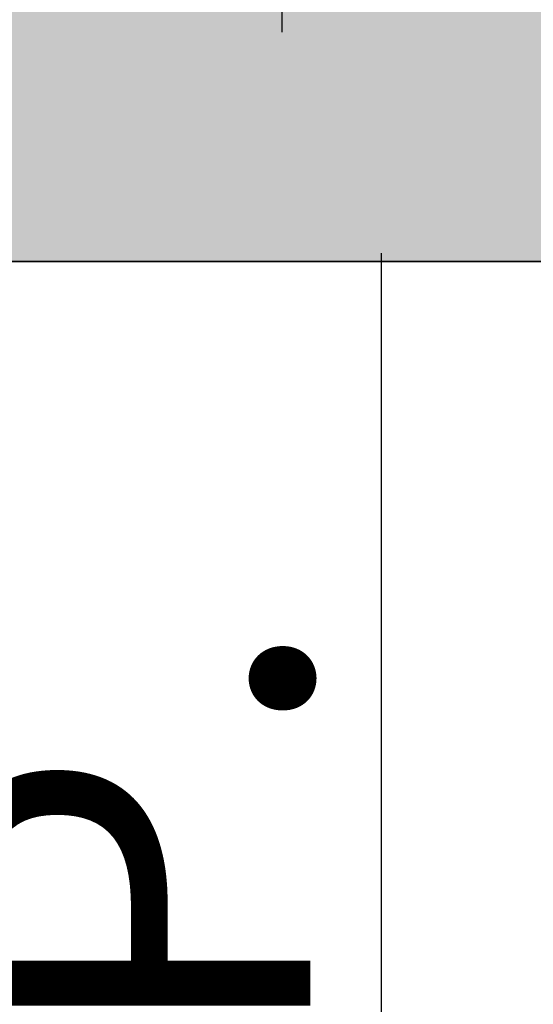
# Model space of a CAD drawing. Units: inches. Extents: x 2083 to 3317, y 1141 to 2115.
# Tile 124 of 256: x 3102 to 3120, y 1238 to 1271. Entities that reach past the tile are written whole.
import ezdxf

# ---------------------------------------------------------------- set-up
doc = ezdxf.new("R2010")
doc.units = ezdxf.units.IN
doc.layers.add('A-ANNO-DIMS', color=2, linetype='Continuous', lineweight=18)
doc.layers.add('A-WALL', color=7, linetype='Continuous', lineweight=35)
doc.layers.add('A-WALL-PATT', color=251, linetype='Continuous', lineweight=13, true_color=0x636466)
doc.styles.get("Standard").update_dxf_attribs({"font": 'arial.ttf'})
doc.dimstyles.new('ISO-25', dxfattribs={"dimtxt": 12, "dimasz": 12, "dimexe": 1.25, "dimexo": 0.625, "dimtad": 1, "dimlunit": 3, "dimtxsty": 'Standard', "dimcen": 2.5, "dimadec": 0, "dimazin": 0, "dimtfac": 1, "dimtmove": 0, "dimatfit": 3, "dimfxl": 1, "dimarcsym": 0})

# ---------------------------------------------------------------- blocks, each defined once
blk = doc.blocks.new('*D10')
at = {"layer": 'A-ANNO-DIMS', "color": 0, "lineweight": -2, "transparency": 16777216}
for p, q in [((2862.96, 1262.636), (2862.96, 1201.384)), ((3126.96, 1262.636), (3126.96, 1201.384)), ((2874.96, 1202.634), (3114.96, 1202.634))]:
    blk.add_line(p, q, dxfattribs=at)
at = {"layer": 'A-ANNO-DIMS', "color": 0, "transparency": 16777216}
for points in [[(2874.96, 1204.634), (2874.96, 1200.634), (2862.96, 1202.634)], [(3114.96, 1204.634), (3114.96, 1200.634), (3126.96, 1202.634)]]:
    blk.add_solid(points, dxfattribs=at)
at = {"layer": 'Defpoints', "color": 0, "transparency": 16777216}
for p in [(2862.96, 1263.261), (3126.96, 1263.261), (3126.96, 1202.634)]:
    blk.add_point(p, dxfattribs=at)
at = {"layer": 'A-ANNO-DIMS', "color": 0, "transparency": 16777216, "insert": (2994.96, 1209.284), "char_height": 12, "attachment_point": 5}
blk.add_mtext("22'", dxfattribs=at)
blk = doc.blocks.new('*D26')
at = {"layer": 'A-ANNO-DIMS', "color": 0, "lineweight": -2, "transparency": 16777216}
for p, q in [((3088.986, 1274.915), (3088.986, 1270.952)), ((3111.24, 1274.915), (3111.24, 1270.952)), ((3076.986, 1272.202), (2840.262, 1272.202)), ((3111.24, 1272.202), (3088.986, 1272.202)), ((3123.24, 1272.202), (3135.24, 1272.202))]:
    blk.add_line(p, q, dxfattribs=at)
at = {"layer": 'A-ANNO-DIMS', "color": 0, "transparency": 16777216}
for points in [[(3076.986, 1274.202), (3076.986, 1270.202), (3088.986, 1272.202)], [(3123.24, 1274.202), (3123.24, 1270.202), (3111.24, 1272.202)]]:
    blk.add_solid(points, dxfattribs=at)
at = {"layer": 'Defpoints', "color": 0, "transparency": 16777216}
for p in [(3088.986, 1275.54), (3111.24, 1275.54), (3088.986, 1272.202)]:
    blk.add_point(p, dxfattribs=at)
at = {"layer": 'A-ANNO-DIMS', "color": 0, "transparency": 16777216, "insert": (2952.624, 1279.032), "char_height": 12, "attachment_point": 5}
blk.add_mtext('NIGHTSTAND 1\'-10 1/2" TYP.', dxfattribs=at)
blk = doc.blocks.new('*D27')
at = {"layer": 'A-ANNO-DIMS', "color": 0, "lineweight": -2, "transparency": 16777216}
for p, q in [((3114.578, 1309.794), (3114.578, 1321.794)), ((3111.865, 1297.794), (3115.828, 1297.794)), ((3114.578, 1297.794), (3114.578, 1275.54)), ((3111.865, 1275.54), (3115.828, 1275.54)), ((3114.578, 1263.54), (3114.578, 1140.989))]:
    blk.add_line(p, q, dxfattribs=at)
at = {"layer": 'A-ANNO-DIMS', "color": 0, "transparency": 16777216}
for points in [[(3112.578, 1309.794), (3116.578, 1309.794), (3114.578, 1297.794)], [(3112.578, 1263.54), (3116.578, 1263.54), (3114.578, 1275.54)]]:
    blk.add_solid(points, dxfattribs=at)
at = {"layer": 'Defpoints', "color": 0, "transparency": 16777216}
for p in [(3111.24, 1297.794), (3111.24, 1275.54), (3114.578, 1275.54)]:
    blk.add_point(p, dxfattribs=at)
at = {"layer": 'A-ANNO-DIMS', "color": 0, "transparency": 16777216, "insert": (3107.749, 1196.264), "char_height": 12, "attachment_point": 5, "rotation": 90}
blk.add_mtext('1\'-10 1/2" TYP.', dxfattribs=at)
blk = doc.blocks.new('*D34')
at = {"layer": 'A-ANNO-DIMS', "color": 0, "lineweight": -2, "transparency": 16777216}
for p, q in [((2226.96, 1262.636), (2226.96, 1209.661)), ((3126.96, 1262.636), (3126.96, 1209.661)), ((2238.96, 1210.911), (3114.96, 1210.911))]:
    blk.add_line(p, q, dxfattribs=at)
at = {"layer": 'A-ANNO-DIMS', "color": 0, "transparency": 16777216}
for points in [[(2238.96, 1212.911), (2238.96, 1208.911), (2226.96, 1210.911)], [(3114.96, 1212.911), (3114.96, 1208.911), (3126.96, 1210.911)]]:
    blk.add_solid(points, dxfattribs=at)
at = {"layer": 'Defpoints', "color": 0, "transparency": 16777216}
for p in [(2226.96, 1263.261), (3126.96, 1263.261), (3126.96, 1210.911)]:
    blk.add_point(p, dxfattribs=at)
at = {"layer": 'A-ANNO-DIMS', "color": 0, "transparency": 16777216, "insert": (2676.96, 1217.663), "char_height": 12, "attachment_point": 5}
blk.add_mtext('75\'-0"', dxfattribs=at)

msp = doc.modelspace()

# ---------------------------------------------------------------- hatches: boundary and pattern name
at = {"layer": 'A-WALL-PATT'}
h = msp.add_hatch(color=256, dxfattribs=at)
h.dxf.hatch_style = 1
h.paths.add_polyline_path([(3126.96, 2020.761), (2748.96, 2020.761), (2604.96, 2020.761), (2226.96, 2020.761), (2226.96, 1702.761), (2466.96, 1702.761), (2466.96, 1582.761), (2418.96, 1582.761), (2418.96, 1477.761), (2226.96, 1477.761), (2226.96, 1263.261), (2544.96, 1263.261), (2544.96, 1411.761), (2604.96, 1411.761), (2685.96, 1411.761), (2685.96, 1420.761), (2604.96, 1420.761), (2604.96, 1573.761), (2604.96, 1702.761), (2604.96, 2011.761), (2748.96, 2011.761), (2748.96, 1702.761), (2862.96, 1702.761), (2862.96, 1621.761), (2871.96, 1621.761), (2871.96, 1702.761), (2883.96, 1702.761), (2883.96, 1706.939, -0.026459), (2883.96, 1711.761), (2757.96, 1711.761), (2757.96, 1807.761), (2787.96, 1807.761), (2787.96, 1812.261), (2757.96, 1812.261), (2757.96, 2011.761), (2877.96, 2011.761), (2877.96, 1812.261), (2847.96, 1812.261), (2847.96, 1807.761), (2889.836, 1807.761), (2889.836, 1812.261), (2882.46, 1812.261), (2882.46, 2011.761), (3117.96, 2011.761), (3117.96, 1812.261), (2937.836, 1812.261), (2937.836, 1807.761), (2995.71, 1807.761), (2995.71, 1796.118), (3000.21, 1796.118), (3000.21, 1807.761), (3117.96, 1807.761), (3117.96, 1711.761), (3000.21, 1711.761), (3000.21, 1760.118), (2998.573, 1760.118, -0.020711), (2995.71, 1760.118), (2995.71, 1711.761), (2931.96, 1711.761), (2931.96, 1702.761), (3126.96, 1702.761)])
h.paths.add_polyline_path([(2471.46, 2011.761), (2471.46, 1810.011), (2462.717, 1810.011), (2462.717, 1805.511), (2505.96, 1805.511), (2505.96, 1810.011), (2475.96, 1810.011), (2475.96, 2011.761), (2595.96, 2011.761), (2595.96, 1810.011), (2565.96, 1810.011), (2565.96, 1805.511), (2595.96, 1805.511), (2595.96, 1711.761), (2235.96, 1711.761), (2235.96, 1805.511), (2353.71, 1805.511), (2353.71, 1796.054), (2358.21, 1796.054), (2358.21, 1805.511), (2414.717, 1805.511), (2414.717, 1810.011), (2235.96, 1810.011), (2235.96, 2011.761)], flags=16)
h.paths.add_polyline_path([(2270.205, 1994.61), (2270.205, 1970.61), (2246.205, 1970.61), (2246.205, 1994.61)], flags=0)
edge = h.paths.add_edge_path(flags=0)
edge.add_ellipse((2332.027, 1899.798), major_axis=(-3.043, 3.043), ratio=0.168252, start_angle=-161.3322, end_angle=-156.3071, ccw=False)
edge.add_ellipse((2333.082, 1898.744), major_axis=(-1.055, 1.055), ratio=0.453532, start_angle=-123.371, end_angle=-94.1591)
edge = h.paths.add_edge_path(flags=0)
edge.add_ellipse((2332.027, 1968.876), major_axis=(3.043, 3.043), ratio=0.168252, start_angle=18.6678, end_angle=23.6929)
edge.add_spline(control_points=[(2332.926, 1970.691), (2332.227, 1970.336), (2330.894, 1969.659), (2328.413, 1970.932), (2327.204, 1967.749), (2324.71, 1969.956), (2322.533, 1967.012), (2320.013, 1971.296), (2317.68, 1968.158), (2316.041, 1967.102), (2315.427, 1966.81)], knot_values=[0, 0, 0, 0, 2.267059, 4.324559, 6.685584, 8.878641, 11.121502, 14.300359, 17.755284, 19.732645, 19.732645, 19.732645, 19.732645], degree=3, periodic=0)
edge.add_ellipse((2332.027, 1968.876), major_axis=(3.043, 3.043), ratio=0.168252, start_angle=18.6678, end_angle=23.6929, ccw=False)
edge.add_ellipse((2333.082, 1969.931), major_axis=(1.055, 1.055), ratio=0.453532, start_angle=56.629, end_angle=85.8409, ccw=False)
edge = h.paths.add_edge_path(flags=0)
edge.add_spline(control_points=[(2296.428, 1967.988), (2293.628, 1965.336), (2287.704, 1959.727), (2299.744, 1949.996), (2294.533, 1935.669), (2290.573, 1920.604), (2293.394, 1909.974), (2296.185, 1904.967)], knot_values=[0.099185, 0.099185, 0.099185, 0.099185, 0.345301, 0.619822, 0.982653, 1.386093, 1.810555, 1.810555, 1.810555, 1.810555], degree=3, periodic=0)
edge.add_spline(control_points=[(2296.185, 1904.967), (2297.384, 1902.619), (2298.001, 1901.949), (2298.553, 1901.468)], knot_values=[0.006246, 0.006246, 0.006246, 0.006246, 0.055476, 0.055476, 0.055476, 0.055476], degree=3, periodic=0)
edge.add_spline(control_points=[(2298.553, 1901.468), (2297.259, 1900.923), (2295.225, 1900.232), (2293.06, 1900.614), (2292.101, 1900.788), (2292.09, 1900.791)], knot_values=[0.312835, 0.312835, 0.312835, 0.312835, 0.40178, 0.474987, 0.475903, 0.475903, 0.475903, 0.475903], degree=3, periodic=0)
edge.add_arc((2292.794, 1904.664), 3.937, 215.4209, 259.6982, ccw=False)
edge.add_spline(control_points=[(2289.585, 1902.382), (2289.477, 1902.535), (2289.368, 1902.688), (2289.261, 1902.841)], knot_values=[0.102872, 0.102872, 0.102872, 0.102872, 0.116896, 0.116896, 0.116896, 0.116896], degree=3, periodic=0)
edge.add_spline(control_points=[(2289.261, 1902.841), (2288.687, 1902.55), (2287.64, 1902.02), (2285.881, 1901.874), (2283.853, 1901.504), (2281.72, 1899.711), (2278.467, 1899.493), (2276.157, 1901.883), (2272.259, 1899.804), (2267.778, 1901.843), (2262.244, 1900.184), (2257.415, 1901.782), (2254.318, 1900.726), (2253.178, 1900.337)], knot_values=[0, 0, 0, 0, 1.907977, 3.477176, 5.261074, 7.972851, 11.680248, 13.717921, 16.939592, 22.789562, 27.502503, 33.595215, 37.145618, 37.145618, 37.145618, 37.145618], degree=3, periodic=0)
edge.add_line((2253.178, 1900.337), (2250.244, 1902.841))
edge.add_line((2250.244, 1902.841), (2250.244, 1965.833))
edge.add_line((2250.244, 1965.833), (2253.178, 1968.337))
edge.add_spline(control_points=[(2253.178, 1968.337), (2254.318, 1967.948), (2257.415, 1966.892), (2262.244, 1968.49), (2267.778, 1966.831), (2271.527, 1968.537), (2273.876, 1967.828), (2274.207, 1967.728)], knot_values=[0, 0, 0, 0, 0.09018, 0.244935, 0.364644, 0.513233, 0.537855, 0.537855, 0.537855, 0.537855], degree=3, periodic=0)
edge.add_arc((2274.353, 1963.793), 3.937, 72.0511, 92.1279, ccw=False)
edge.add_arc((2281.297, 1985.23), 18.596, 252.0511, 288.5657)
edge.add_arc((2292.317, 1956.029), 12.646, 71.0268, 113.7782, ccw=False)
edge = h.paths.add_edge_path(flags=0)
edge.add_spline(control_points=[(2274.899, 1951.856), (2275.066, 1951.617), (2275.233, 1951.377), (2275.398, 1951.136)], knot_values=[1.409916, 1.409916, 1.409916, 1.409916, 1.43159, 1.43159, 1.43159, 1.43159], degree=3, periodic=0)
edge.add_spline(control_points=[(2275.398, 1951.136), (2275.792, 1950.562), (2276.179, 1949.984), (2276.546, 1949.397)], knot_values=[1.358238, 1.358238, 1.358238, 1.358238, 1.409916, 1.409916, 1.409916, 1.409916], degree=3, periodic=0)
edge.add_line((2276.546, 1949.397), (2277.437, 1947.862))
edge.add_spline(control_points=[(2277.437, 1947.862), (2276.304, 1945.673), (2274.64, 1942.427), (2274.632, 1938.094), (2272.799, 1930.852), (2274.356, 1943.897), (2275.948, 1947.923), (2276.546, 1949.397)], knot_values=[0.005632, 0.005632, 0.005632, 0.005632, 0.186014, 0.266002, 0.357087, 0.59639, 0.739732, 0.739732, 0.739732, 0.739732], degree=3, periodic=0)
edge.add_spline(control_points=[(2276.546, 1949.397), (2276.179, 1949.984), (2275.792, 1950.562), (2275.398, 1951.136)], knot_values=[1.358238, 1.358238, 1.358238, 1.358238, 1.409916, 1.409916, 1.409916, 1.409916], degree=3, periodic=0)
edge.add_spline(control_points=[(2275.398, 1951.136), (2274.943, 1950.08), (2274.208, 1948.025), (2273.935, 1944.851), (2272.469, 1937.627), (2273.466, 1945.696), (2274.701, 1951.059), (2274.899, 1951.856)], knot_values=[0.104364, 0.104364, 0.104364, 0.104364, 0.189636, 0.269624, 0.36071, 0.600013, 0.644622, 0.644622, 0.644622, 0.644622], degree=3, periodic=0)
h.paths.add_polyline_path([(2269.168, 1963.128, -0.357527), (2268.171, 1960.976, -0.092561), (2268.171, 1939.436, -0.357527), (2269.168, 1937.285, -0.357527), (2267.016, 1938.282, -0.164785), (2254.686, 1938.282, -0.357527), (2252.534, 1937.285, -0.357527), (2253.531, 1939.436, -0.092561), (2253.531, 1960.976, -0.357527), (2252.534, 1963.128, -0.357527), (2254.686, 1962.131, -0.164785), (2267.016, 1962.131, -0.357527)], flags=0)
h.paths.add_polyline_path([(2248.874, 1967.802), (2248.874, 1957.028), (2249.458, 1957.028), (2249.458, 1911.647), (2248.874, 1911.647), (2248.874, 1900.873), (2246.512, 1900.873, 0.197327), (2244.15, 1902.457), (2244.15, 1966.218, 0.197327), (2246.512, 1967.802)], flags=0)
h.paths.add_polyline_path([(2269.168, 1931.389, -0.357527), (2268.171, 1929.238, -0.092561), (2268.171, 1907.698, -0.357527), (2269.168, 1905.547, -0.357527), (2267.016, 1906.544, -0.164785), (2254.686, 1906.544, -0.357527), (2252.534, 1905.547, -0.357527), (2253.531, 1907.698, -0.092561), (2253.531, 1929.238, -0.357527), (2252.534, 1931.389, -0.357527), (2254.686, 1930.392, -0.164785), (2267.016, 1930.392, -0.357527)], flags=0)
edge = h.paths.add_edge_path(flags=0)
edge.add_spline(control_points=[(2276.197, 1906.724), (2276.168, 1909.029), (2276.114, 1913.372), (2270.598, 1924.925), (2273.905, 1919.013), (2275.922, 1916.262), (2275.475, 1912.402), (2277.258, 1910.381), (2276.696, 1908.225), (2276.646, 1906.813), (2276.618, 1906.008)], knot_values=[0, 0, 0, 0, 8.61026, 16.221274, 18.843057, 23.804898, 27.440828, 29.356102, 31.203478, 33.650687, 33.650687, 33.650687, 33.650687], degree=3, periodic=0)
edge.add_spline(control_points=[(2276.618, 1906.008), (2276.623, 1905.624), (2276.498, 1904.629), (2275.442, 1903.855), (2274.937, 1903.08), (2274.859, 1902.841)], knot_values=[0.156488, 0.156488, 0.156488, 0.156488, 0.184398, 0.231376, 0.250598, 0.250598, 0.250598, 0.250598], degree=3, periodic=0)
edge.add_line((2274.859, 1902.841), (2276.506, 1902.841))
edge.add_spline(control_points=[(2276.506, 1902.841), (2276.788, 1903.085), (2277.665, 1904.125), (2278.25, 1904.341), (2277.654, 1908.527), (2278.156, 1906.228), (2278.1, 1905.286), (2278.847, 1904.069), (2277.857, 1903.415), (2277.874, 1902.991), (2277.904, 1902.841)], knot_values=[0.059574, 0.059574, 0.059574, 0.059574, 0.080753, 0.103741, 0.16972, 0.176036, 0.207137, 0.240474, 0.262341, 0.27366, 0.27366, 0.27366, 0.27366], degree=3, periodic=0)
edge.add_line((2277.904, 1902.841), (2280.03, 1902.841))
edge.add_spline(control_points=[(2280.03, 1902.841), (2279.888, 1903.088), (2279.499, 1903.982), (2280.152, 1905.939), (2278.104, 1909.658), (2279.762, 1907.185), (2280.328, 1904.875), (2280.485, 1903.49), (2281.463, 1903.249), (2281.758, 1902.936), (2281.834, 1902.841)], knot_values=[0.013856, 0.013856, 0.013856, 0.013856, 0.034874, 0.088867, 0.107879, 0.126738, 0.158714, 0.193757, 0.217487, 0.226722, 0.226722, 0.226722, 0.226722], degree=3, periodic=0)
edge.add_spline(control_points=[(2281.834, 1902.841), (2281.788, 1902.827), (2281.647, 1902.783), (2281.396, 1902.859), (2281.088, 1902.985), (2280.721, 1903.061), (2280.333, 1903.026), (2280.125, 1902.899), (2280.03, 1902.841)], knot_values=[0, 0, 0, 0, 0.14413, 0.435517, 0.749276, 1.153046, 1.548371, 1.878348, 1.878348, 1.878348, 1.878348], degree=3, periodic=0)
edge.add_line((2280.03, 1902.841), (2277.904, 1902.841))
edge.add_spline(control_points=[(2277.904, 1902.841), (2277.893, 1902.796), (2277.865, 1902.68), (2277.607, 1902.687), (2277.274, 1902.801), (2276.838, 1902.62), (2276.584, 1902.789), (2276.506, 1902.841)], knot_values=[0, 0, 0, 0, 0.127189, 0.326199, 0.628009, 1.24357, 1.515331, 1.515331, 1.515331, 1.515331], degree=3, periodic=0)
edge.add_line((2276.506, 1902.841), (2274.859, 1902.841))
edge.add_spline(control_points=[(2274.859, 1902.841), (2274.814, 1902.899), (2274.725, 1903.013), (2274.493, 1903.119), (2274.244, 1902.961), (2273.937, 1903.185), (2273.614, 1902.983), (2273.408, 1902.883), (2273.322, 1902.841)], knot_values=[0, 0, 0, 0, 0.21843, 0.436957, 0.687977, 0.990379, 1.398396, 1.69185, 1.69185, 1.69185, 1.69185], degree=3, periodic=0)
edge.add_spline(control_points=[(2273.322, 1902.841), (2273.617, 1903.446), (2274.274, 1904.538), (2276.027, 1904.574), (2276.207, 1906.584), (2276.197, 1906.724)], knot_values=[0.012227, 0.012227, 0.012227, 0.012227, 0.059472, 0.106218, 0.134458, 0.134458, 0.134458, 0.134458], degree=3, periodic=0)
h.paths.add_polyline_path([(2270.776, 1897.79), (2270.776, 1873.79), (2246.776, 1873.79), (2246.776, 1897.79)], flags=0)
h.paths.add_polyline_path([(2353.71, 1760.005), (2353.71, 1760.054), (2358.21, 1760.054, -0.033729)], flags=0)
h.paths.add_polyline_path([(2321.819, 1737.529), (2341.995, 1737.529, -0.414214), (2343.203, 1736.321), (2343.203, 1721.021, -0.414214), (2341.995, 1719.813), (2321.819, 1719.813, -0.414214), (2320.611, 1721.021), (2320.611, 1736.321, -0.414214)], flags=0)
h.paths.add_polyline_path([(2324.235, 1736.321), (2339.579, 1736.321, -0.414214), (2341.995, 1733.905), (2341.995, 1725.45, -0.414214), (2339.579, 1723.034), (2333.681, 1723.034), (2333.845, 1722.045, -0.870646), (2335.425, 1721.826, -0.767327), (2333.923, 1721.423), (2331.291, 1721.423, -0.767327), (2329.788, 1721.826, -0.870646), (2331.368, 1722.045), (2331.533, 1723.034), (2324.235, 1723.034, -0.414214), (2321.819, 1725.45), (2321.819, 1733.905, -0.414214)], flags=0)
h.paths.add_polyline_path([(2570.484, 1928.615), (2589.684, 1928.615), (2590.169, 1928.615), (2590.169, 1904.993), (2570.484, 1904.993)], flags=0)
h.paths.add_polyline_path([(2574.447, 1927.264, -1), (2572.829, 1927.264, -1)], flags=0)
h.paths.add_polyline_path([(2573.09, 1926.941), (2573.925, 1927.776), (2574.148, 1927.553), (2573.313, 1926.718)], flags=0)
h.paths.add_polyline_path([(2578.779, 1919.73, -1), (2571.592, 1919.73, -1)], flags=0)
h.paths.add_polyline_path([(2578.385, 1919.73, -1), (2571.985, 1919.73, -1)], flags=0)
h.paths.add_polyline_path([(2331.596, 1729.476, -1), (2333.618, 1729.476, -1)], flags=0)
h.paths.add_polyline_path([(2578.034, 1927.264, -1), (2576.416, 1927.264, -1)], flags=0)
h.paths.add_polyline_path([(2576.689, 1927.531), (2576.912, 1927.754), (2577.747, 1926.919), (2577.524, 1926.696)], flags=0)
h.paths.add_polyline_path([(2578.139, 1909.86, -1), (2572.232, 1909.86, -1)], flags=0)
h.paths.add_polyline_path([(2577.745, 1909.86, -1), (2572.625, 1909.86, -1)], flags=0)
h.paths.add_polyline_path([(2583.798, 1927.264, -1), (2582.179, 1927.264, -1)], flags=0)
h.paths.add_polyline_path([(2582.719, 1927.754), (2583.554, 1926.919), (2583.331, 1926.696), (2582.496, 1927.531)], flags=0)
h.paths.add_polyline_path([(2582.496, 1927.531), (2582.719, 1927.754), (2583.554, 1926.919), (2583.331, 1926.696)], flags=0)
h.paths.add_polyline_path([(2587.739, 1920.53, -1), (2581.832, 1920.53, -1)], flags=0)
h.paths.add_polyline_path([(2587.345, 1920.53, -1), (2582.225, 1920.53, -1)], flags=0)
h.paths.add_polyline_path([(2587.385, 1927.264, -1), (2585.766, 1927.264, -1)], flags=0)
h.paths.add_polyline_path([(2586.082, 1926.98), (2586.917, 1927.815), (2587.14, 1927.593), (2586.305, 1926.758)], flags=0)
h.paths.add_polyline_path([(2588.379, 1910.66, -1), (2581.192, 1910.66, -1)], flags=0)
h.paths.add_polyline_path([(2587.985, 1910.66, -1), (2581.585, 1910.66, -1)], flags=0)
h.paths.add_polyline_path([(2417.168, 1729.478), (2437.344, 1729.478, -0.414214), (2438.552, 1728.27), (2438.552, 1712.969, -0.414214), (2437.344, 1711.761), (2417.168, 1711.761, -0.414214), (2415.96, 1712.969), (2415.96, 1728.27, -0.414214)], flags=0)
h.paths.add_polyline_path([(2419.584, 1728.27), (2434.928, 1728.27, -0.414214), (2437.344, 1725.854), (2437.344, 1717.398, -0.414214), (2434.928, 1714.983), (2429.029, 1714.983), (2429.194, 1713.994, -0.870646), (2430.774, 1713.775, -0.767327), (2429.271, 1713.372), (2426.64, 1713.372, -0.767327), (2425.137, 1713.775, -0.870646), (2426.717, 1713.994), (2426.882, 1714.983), (2419.584, 1714.983, -0.414214), (2417.168, 1717.398), (2417.168, 1725.854, -0.414214)], flags=0)
h.paths.add_polyline_path([(2419.584, 1728.27), (2434.928, 1728.27, -0.414214), (2437.344, 1725.854), (2437.344, 1717.398, -0.414214), (2434.928, 1714.983), (2429.029, 1714.983), (2428.358, 1719.009), (2427.553, 1719.009), (2426.882, 1714.983), (2419.584, 1714.983, -0.414214), (2417.168, 1717.398), (2417.168, 1725.854, -0.414214)], flags=0)
h.paths.add_polyline_path([(2426.944, 1721.425, -1), (2428.967, 1721.425, -1)], flags=0)
h.paths.add_polyline_path([(2475.96, 1702.761), (2595.96, 1702.761), (2595.96, 1582.761), (2475.96, 1582.761)], flags=16)
h.paths.add_polyline_path([(2427.96, 1573.761), (2595.96, 1573.761), (2595.96, 1468.761), (2595.96, 1420.761), (2384.46, 1420.761), (2384.46, 1468.761), (2427.96, 1468.761)], flags=16)
h.paths.add_polyline_path([(2379.96, 1468.761), (2379.96, 1420.761), (2235.96, 1420.761), (2235.96, 1468.761)], flags=16)
h.paths.add_polyline_path([(2317.816, 1466.696), (2337.992, 1466.696, -0.414214), (2339.2, 1465.488), (2339.2, 1450.187, -0.414214), (2337.992, 1448.979), (2317.816, 1448.979, -0.414214), (2316.608, 1450.187), (2316.608, 1465.488, -0.414214)], flags=0)
h.paths.add_polyline_path([(2320.232, 1465.488), (2335.576, 1465.488, -0.414214), (2337.992, 1463.072), (2337.992, 1454.616, -0.414214), (2335.576, 1452.2), (2329.677, 1452.2), (2329.842, 1451.212, -0.870646), (2331.422, 1450.992, -0.767327), (2329.92, 1450.59), (2327.288, 1450.59, -0.767327), (2325.785, 1450.992, -0.870646), (2327.365, 1451.212), (2327.53, 1452.2), (2320.232, 1452.2, -0.414214), (2317.816, 1454.616), (2317.816, 1463.072, -0.414214)], flags=0)
h.paths.add_polyline_path([(2320.232, 1465.488), (2335.576, 1465.488, -0.414214), (2337.992, 1463.072), (2337.992, 1454.616, -0.414214), (2335.576, 1452.2), (2329.677, 1452.2), (2329.006, 1456.227), (2328.201, 1456.227), (2327.53, 1452.2), (2320.232, 1452.2, -0.414214), (2317.816, 1454.616), (2317.816, 1463.072, -0.414214)], flags=0)
h.paths.add_polyline_path([(2327.593, 1458.643, -1), (2329.615, 1458.643, -1)], flags=0)
h.paths.add_polyline_path([(2244.412, 1433.34), (2241.921, 1433.34, -0.414214), (2240.018, 1435.244), (2240.018, 1440.953, -0.414211), (2241.921, 1442.856), (2244.412, 1442.856, -1.976472)], flags=0)
h.paths.add_polyline_path([(2245.357, 1434.398, -0.414214), (2245.357, 1441.799, -2.144098)], flags=0)
h.paths.add_polyline_path([(2535.96, 1416.261), (2535.96, 1272.261), (2235.96, 1272.261), (2235.96, 1416.261)], flags=16)
h.paths.add_polyline_path([(2260.12, 1384.293), (2260.12, 1362.039), (2237.865, 1362.039), (2237.865, 1384.293)], flags=0)
edge = h.paths.add_edge_path(flags=0)
edge.add_line((2318.252, 1362.093), (2318.146, 1362.001))
edge.add_ellipse((2317.445, 1360.431), major_axis=(2.822, 2.822), ratio=0.168252, start_angle=18.6678, end_angle=20.9481, ccw=False)
edge.add_ellipse((2318.423, 1361.409), major_axis=(0.978, 0.978), ratio=0.453532, start_angle=56.629, end_angle=70.2262, ccw=False)
edge = h.paths.add_edge_path(flags=0)
edge.add_line((2319.107, 1295.571), (2319.015, 1295.677))
edge.add_ellipse((2317.445, 1296.378), major_axis=(-2.822, 2.822), ratio=0.168252, start_angle=-161.3322, end_angle=-159.0519, ccw=False)
edge.add_ellipse((2318.423, 1295.4), major_axis=(-0.978, 0.978), ratio=0.453532, start_angle=-123.371, end_angle=-109.7738)
edge = h.paths.add_edge_path(flags=0)
edge.add_spline(control_points=[(2284.21, 1301.17), (2284.581, 1300.445), (2284.891, 1299.892), (2285.16, 1299.461)], knot_values=[0.039066, 0.039066, 0.039066, 0.039066, 0.055476, 0.055476, 0.055476, 0.055476], degree=3, periodic=0)
edge.add_line((2285.16, 1299.461), (2284.21, 1301.17))
edge = h.paths.add_edge_path(flags=0)
edge.add_line((2280.412, 1297.298), (2283.37, 1297.036))
edge.add_line((2283.37, 1297.036), (2286.406, 1297.926))
edge.add_spline(control_points=[(2286.406, 1297.926), (2285.305, 1297.463), (2284.345, 1297.129), (2283.37, 1297.036)], knot_values=[0.394369, 0.394369, 0.394369, 0.394369, 0.475903, 0.475903, 0.475903, 0.475903], degree=3, periodic=0)
edge.add_spline(control_points=[(2283.37, 1297.036), (2283.281, 1297.028), (2282.316, 1296.957), (2281.313, 1297.134), (2280.423, 1297.296), (2280.412, 1297.298)], knot_values=[0.312835, 0.312835, 0.312835, 0.312835, 0.320246, 0.393453, 0.394369, 0.394369, 0.394369, 0.394369], degree=3, periodic=0)
edge = h.paths.add_edge_path(flags=0)
edge.add_line((2284.436, 1359.607), (2280.446, 1355.328))
edge.add_line((2280.446, 1355.328), (2279.58, 1351.018))
edge.add_line((2279.58, 1351.018), (2282.413, 1346.58))
edge.add_spline(control_points=[(2282.413, 1346.58), (2283.153, 1345.589), (2284.253, 1344.029), (2284.801, 1342.387), (2284.935, 1341.806)], knot_values=[1.240098, 1.240098, 1.240098, 1.240098, 1.332892, 1.382712, 1.382712, 1.382712, 1.382712], degree=3, periodic=0)
edge.add_spline(control_points=[(2284.935, 1341.806), (2285.319, 1340.141), (2285.233, 1338.409), (2284.91, 1336.654)], knot_values=[1.097484, 1.097484, 1.097484, 1.097484, 1.240098, 1.240098, 1.240098, 1.240098], degree=3, periodic=0)
edge.add_spline(control_points=[(2284.91, 1336.654), (2284.587, 1334.899), (2284.027, 1333.12), (2283.463, 1331.361)], knot_values=[0.95487, 0.95487, 0.95487, 0.95487, 1.097484, 1.097484, 1.097484, 1.097484], degree=3, periodic=0)
edge.add_line((2283.463, 1331.361), (2281.89, 1326.153))
edge.add_line((2281.89, 1326.153), (2280.756, 1321.056))
edge.add_line((2280.756, 1321.056), (2280.299, 1316.002))
edge.add_line((2280.299, 1316.002), (2280.716, 1310.95))
edge.add_line((2280.716, 1310.95), (2282.028, 1305.972))
edge.add_line((2282.028, 1305.972), (2284.21, 1301.17))
edge.add_spline(control_points=[(2284.21, 1301.17), (2283.341, 1302.73), (2282.612, 1304.336), (2282.028, 1305.972)], knot_values=[0.099185, 0.099185, 0.099185, 0.099185, 0.241799, 0.241799, 0.241799, 0.241799], degree=3, periodic=0)
edge.add_spline(control_points=[(2282.028, 1305.972), (2281.444, 1307.608), (2281.005, 1309.273), (2280.716, 1310.95)], knot_values=[0.241799, 0.241799, 0.241799, 0.241799, 0.384413, 0.384413, 0.384413, 0.384413], degree=3, periodic=0)
edge.add_spline(control_points=[(2280.716, 1310.95), (2280.433, 1312.588), (2280.289, 1314.277), (2280.299, 1315.962), (2280.299, 1316.002)], knot_values=[0.384413, 0.384413, 0.384413, 0.384413, 0.523647, 0.527028, 0.527028, 0.527028, 0.527028], degree=3, periodic=0)
edge.add_spline(control_points=[(2280.299, 1316.002), (2280.312, 1317.687), (2280.478, 1319.368), (2280.756, 1321.056)], knot_values=[0.527028, 0.527028, 0.527028, 0.527028, 0.669642, 0.669642, 0.669642, 0.669642], degree=3, periodic=0)
edge.add_spline(control_points=[(2280.756, 1321.056), (2281.035, 1322.744), (2281.426, 1324.44), (2281.89, 1326.153)], knot_values=[0.669642, 0.669642, 0.669642, 0.669642, 0.812256, 0.812256, 0.812256, 0.812256], degree=3, periodic=0)
edge.add_spline(control_points=[(2281.89, 1326.153), (2282.264, 1327.533), (2282.788, 1329.262), (2283.353, 1331.018), (2283.463, 1331.361)], knot_values=[0.812256, 0.812256, 0.812256, 0.812256, 0.927087, 0.95487, 0.95487, 0.95487, 0.95487], degree=3, periodic=0)
edge.add_line((2283.463, 1331.361), (2284.91, 1336.654))
edge.add_line((2284.91, 1336.654), (2284.935, 1341.806))
edge.add_line((2284.935, 1341.806), (2282.413, 1346.58))
edge.add_spline(control_points=[(2282.413, 1346.58), (2281.275, 1348.104), (2280.078, 1349.57), (2279.58, 1351.018)], knot_values=[1.382712, 1.382712, 1.382712, 1.382712, 1.525326, 1.525326, 1.525326, 1.525326], degree=3, periodic=0)
edge.add_spline(control_points=[(2279.58, 1351.018), (2279.443, 1351.415), (2279.136, 1352.857), (2279.735, 1354.29), (2280.446, 1355.328)], knot_values=[1.525326, 1.525326, 1.525326, 1.525326, 1.564439, 1.667941, 1.667941, 1.667941, 1.667941], degree=3, periodic=0)
edge.add_spline(control_points=[(2280.446, 1355.328), (2281.426, 1356.758), (2282.931, 1358.183), (2284.436, 1359.607)], knot_values=[1.667941, 1.667941, 1.667941, 1.667941, 1.810555, 1.810555, 1.810555, 1.810555], degree=3, periodic=0)
edge.add_arc((2280.623, 1348.518), 11.726, 71.0268, 113.7782)
edge.add_arc((2270.405, 1375.595), 17.244, 252.0511, 288.5657, ccw=False)
edge.add_arc((2263.966, 1355.718), 3.651, 72.0511, 92.1279)
edge.add_arc((2263.966, 1355.718), 3.651, 92.1279, 177.9851)
edge.add_spline(control_points=[(2260.318, 1355.846), (2260.26, 1354.221), (2260.551, 1350.187), (2262.999, 1346.766), (2264.473, 1344.649)], knot_values=[1.43159, 1.43159, 1.43159, 1.43159, 1.564144, 1.770695, 1.770695, 1.770695, 1.770695], degree=3, periodic=0)
edge.add_line((2264.473, 1344.649), (2264.936, 1343.983))
edge.add_spline(control_points=[(2263.801, 1340.248), (2263.843, 1340.514), (2264.067, 1341.756), (2264.513, 1343.002), (2264.935, 1343.981)], knot_values=[0.53657, 0.53657, 0.53657, 0.53657, 0.559349, 0.644622, 0.644622, 0.644622, 0.644622], degree=3, periodic=0)
edge.add_spline(control_points=[(2264.935, 1343.981), (2265.118, 1343.715), (2265.299, 1343.448), (2265.477, 1343.179)], knot_values=[1.384077, 1.384077, 1.384077, 1.384077, 1.409916, 1.409916, 1.409916, 1.409916], degree=3, periodic=0)
edge.add_spline(control_points=[(2265.477, 1343.179), (2265.655, 1342.911), (2265.829, 1342.641), (2265.999, 1342.369)], knot_values=[1.358238, 1.358238, 1.358238, 1.358238, 1.384077, 1.384077, 1.384077, 1.384077], degree=3, periodic=0)
edge.add_line((2265.999, 1342.369), (2266.826, 1340.946))
edge.add_spline(control_points=[(2266.826, 1340.946), (2268.894, 1337.09), (2271.398, 1325.843), (2270.516, 1310.569), (2275.919, 1301.861), (2277.79, 1299.199)], knot_values=[0.116896, 0.116896, 0.116896, 0.116896, 0.472987, 1.050969, 1.313793, 1.313793, 1.313793, 1.313793], degree=3, periodic=0)
edge.add_spline(control_points=[(2277.79, 1299.199), (2277.839, 1299.128), (2277.889, 1299.057), (2277.94, 1298.987)], knot_values=[0.109884, 0.109884, 0.109884, 0.109884, 0.116896, 0.116896, 0.116896, 0.116896], degree=3, periodic=0)
edge.add_line((2277.94, 1298.987), (2277.789, 1299.199))
edge.add_spline(control_points=[(2277.789, 1299.199), (2277.257, 1298.929), (2276.286, 1298.438), (2275.039, 1298.334), (2274.383, 1298.239), (2274.215, 1298.209)], knot_values=[33.12187, 33.12187, 33.12187, 33.12187, 35.029056, 36.598255, 37.144827, 37.144827, 37.144827, 37.144827], degree=3, periodic=0)
edge.add_line((2274.215, 1298.209), (2273.073, 1297.893))
edge.add_spline(control_points=[(2273.073, 1297.893), (2272.323, 1297.58), (2271.039, 1296.511), (2269.248, 1296.226), (2268.423, 1296.375)], knot_values=[26.532584, 26.532584, 26.532584, 26.532584, 29.198919, 31.839101, 31.839101, 31.839101, 31.839101], degree=3, periodic=0)
edge.add_line((2268.423, 1296.375), (2263.879, 1297.458))
edge.add_spline(control_points=[(2263.879, 1297.458), (2263.556, 1297.359), (2261.86, 1296.839), (2260.239, 1297.282), (2258.933, 1297.516)], knot_values=[15.919551, 15.919551, 15.919551, 15.919551, 16.939592, 21.226067, 21.226067, 21.226067, 21.226067], degree=3, periodic=0)
edge.add_line((2258.933, 1297.516), (2254.055, 1297.329))
edge.add_spline(control_points=[(2254.055, 1297.329), (2253.756, 1297.296), (2252.114, 1297.165), (2250.462, 1297.544), (2249.13, 1297.668)], knot_values=[5.306517, 5.306517, 5.306517, 5.306517, 6.276435, 10.613034, 10.613034, 10.613034, 10.613034], degree=3, periodic=0)
edge.add_line((2249.13, 1297.668), (2244.332, 1296.878))
edge.add_line((2244.332, 1296.878), (2241.611, 1299.199))
edge.add_line((2241.611, 1299.199), (2241.611, 1357.609))
edge.add_line((2241.611, 1357.609), (2244.332, 1359.931))
edge.add_line((2244.332, 1359.931), (2252.729, 1359.543))
edge.add_spline(control_points=[(2252.729, 1359.543), (2252.871, 1359.546), (2253.306, 1359.548), (2253.74, 1359.514), (2254.032, 1359.482)], knot_values=[0.233291, 0.233291, 0.233291, 0.233291, 0.244935, 0.268927, 0.268927, 0.268927, 0.268927], degree=3, periodic=0)
edge.add_line((2254.032, 1359.482), (2259.587, 1359.416))
edge.add_spline(control_points=[(2259.587, 1359.416), (2260.677, 1359.629), (2262.073, 1359.897), (2263.524, 1359.459), (2263.83, 1359.366)], knot_values=[0.422516, 0.422516, 0.422516, 0.422516, 0.513233, 0.537855, 0.537855, 0.537855, 0.537855], degree=3, periodic=0)
edge.add_arc((2263.966, 1355.718), 3.651, 72.0511, 92.1279, ccw=False)
edge.add_arc((2270.405, 1375.595), 17.244, 252.0511, 288.5657)
edge.add_arc((2280.623, 1348.518), 11.726, 71.0268, 113.7782, ccw=False)
h.paths.add_polyline_path([(2240.341, 1359.435), (2240.341, 1349.444), (2240.882, 1349.444), (2240.882, 1307.365), (2240.341, 1307.365), (2240.341, 1297.374), (2238.15, 1297.374, 0.197327), (2235.96, 1298.843), (2235.96, 1357.966, 0.197327), (2238.15, 1359.435)], flags=0)
h.paths.add_polyline_path([(2259.158, 1355.101, -0.357527), (2258.233, 1353.106, -0.092561), (2258.233, 1333.133, -0.357527), (2259.158, 1331.138, -0.357527), (2257.163, 1332.062, -0.164785), (2245.729, 1332.062, -0.357527), (2243.735, 1331.138, -0.357527), (2244.659, 1333.133, -0.092561), (2244.659, 1353.106, -0.357527), (2243.735, 1355.101, -0.357527), (2245.729, 1354.176, -0.164785), (2257.163, 1354.176, -0.357527)], flags=0)
edge = h.paths.add_edge_path(flags=0)
edge.add_line((2265.999, 1342.369), (2266.826, 1340.946))
edge.add_line((2266.826, 1340.946), (2265.308, 1337.814))
edge.add_line((2265.308, 1337.814), (2264.358, 1334.653))
edge.add_line((2264.358, 1334.653), (2264.262, 1333.8))
edge.add_spline(control_points=[(2264.262, 1333.8), (2264.208, 1333.187), (2264.162, 1332.366), (2264.007, 1331.414), (2263.969, 1331.202)], knot_values=[0.464444, 0.464444, 0.464444, 0.464444, 0.516691, 0.531608, 0.531608, 0.531608, 0.531608], degree=3, periodic=0)
edge.add_spline(control_points=[(2263.969, 1331.202), (2263.775, 1330.119), (2263.424, 1328.791), (2263.257, 1328.531), (2263.234, 1328.515)], knot_values=[0.372682, 0.372682, 0.372682, 0.372682, 0.44885, 0.464444, 0.464444, 0.464444, 0.464444], degree=3, periodic=0)
edge.add_spline(control_points=[(2263.234, 1328.515), (2263.096, 1328.42), (2263.131, 1329.301), (2263.275, 1330.616)], knot_values=[0.280919, 0.280919, 0.280919, 0.280919, 0.372682, 0.372682, 0.372682, 0.372682], degree=3, periodic=0)
edge.add_spline(control_points=[(2263.275, 1330.616), (2263.419, 1331.93), (2263.672, 1333.677), (2263.97, 1335.315)], knot_values=[0.189157, 0.189157, 0.189157, 0.189157, 0.280919, 0.280919, 0.280919, 0.280919], degree=3, periodic=0)
edge.add_spline(control_points=[(2263.97, 1335.315), (2264.1, 1336.032), (2264.419, 1337.622), (2264.755, 1338.864), (2264.947, 1339.491)], knot_values=[0.097394, 0.097394, 0.097394, 0.097394, 0.137578, 0.189157, 0.189157, 0.189157, 0.189157], degree=3, periodic=0)
edge.add_spline(control_points=[(2264.947, 1339.491), (2265.29, 1340.606), (2265.644, 1341.494), (2265.999, 1342.369)], knot_values=[0.005632, 0.005632, 0.005632, 0.005632, 0.097394, 0.097394, 0.097394, 0.097394], degree=3, periodic=0)
h.paths.add_polyline_path([(2259.158, 1325.671, -0.357527), (2258.233, 1323.676, -0.092561), (2258.233, 1303.703, -0.357527), (2259.158, 1301.708, -0.357527), (2257.163, 1302.633, -0.164785), (2245.729, 1302.633, -0.357527), (2243.735, 1301.708, -0.357527), (2244.659, 1303.703, -0.092561), (2244.659, 1323.676, -0.357527), (2243.735, 1325.671, -0.357527), (2245.729, 1324.747, -0.164785), (2257.163, 1324.747, -0.357527)], flags=0)
edge = h.paths.add_edge_path(flags=0)
edge.add_spline(control_points=[(2261.709, 1317.311), (2261.679, 1317.418), (2261.762, 1317.389), (2262.491, 1316.09), (2262.962, 1315.301)], knot_values=[14.955861, 14.955861, 14.955861, 14.955861, 16.221274, 18.694826, 18.694826, 18.694826, 18.694826], degree=3, periodic=0)
edge.add_spline(control_points=[(2262.962, 1315.301), (2262.99, 1315.254), (2263.702, 1314.067), (2264.349, 1313.127), (2264.73, 1312.164)], knot_values=[18.694826, 18.694826, 18.694826, 18.694826, 18.843057, 22.433791, 22.433791, 22.433791, 22.433791], degree=3, periodic=0)
edge.add_spline(control_points=[(2264.73, 1312.164), (2264.876, 1311.796), (2265.177, 1310.77), (2265.143, 1309.559), (2265.248, 1308.824)], knot_values=[22.433791, 22.433791, 22.433791, 22.433791, 23.804898, 26.172756, 26.172756, 26.172756, 26.172756], degree=3, periodic=0)
edge.add_line((2265.248, 1308.824), (2265.851, 1307.172))
edge.add_spline(control_points=[(2265.851, 1307.172), (2266.065, 1306.822), (2266.384, 1306.332), (2266.424, 1305.781), (2266.42, 1305.611)], knot_values=[28.062562, 28.062562, 28.062562, 28.062562, 29.356102, 29.911721, 29.911721, 29.911721, 29.911721], degree=3, periodic=0)
edge.add_spline(control_points=[(2266.42, 1305.611), (2266.416, 1305.433), (2266.394, 1305.25), (2266.365, 1305.066)], knot_values=[29.911721, 29.911721, 29.911721, 29.911721, 30.497837, 30.497837, 30.497837, 30.497837], degree=3, periodic=0)
edge.add_line((2266.365, 1305.066), (2266.066, 1302.136))
edge.add_spline(control_points=[(2266.066, 1302.136), (2266.071, 1301.78), (2265.998, 1301.2), (2265.663, 1300.759), (2265.509, 1300.586)], knot_values=[0.156488, 0.156488, 0.156488, 0.156488, 0.184398, 0.203543, 0.203543, 0.203543, 0.203543], degree=3, periodic=0)
edge.add_line((2265.509, 1300.586), (2264.435, 1299.199))
edge.add_line((2264.435, 1299.199), (2265.962, 1299.199))
edge.add_line((2265.962, 1299.199), (2267.336, 1301.175))
edge.add_line((2267.336, 1301.175), (2267.312, 1301.986))
edge.add_spline(control_points=[(2267.312, 1301.986), (2267.261, 1302.862), (2267.16, 1303.737), (2267.271, 1303.326)], knot_values=[0.126229, 0.126229, 0.126229, 0.126229, 0.166617, 0.166617, 0.166617, 0.166617], degree=3, periodic=0)
edge.add_spline(control_points=[(2267.271, 1303.326), (2267.28, 1303.294), (2267.31, 1303.175), (2267.373, 1302.884), (2267.406, 1302.683), (2267.418, 1302.601)], knot_values=[0.166617, 0.166617, 0.166617, 0.166617, 0.16972, 0.176036, 0.180765, 0.180765, 0.180765, 0.180765], degree=3, periodic=0)
edge.add_spline(control_points=[(2267.744, 1300.988), (2267.688, 1301.151), (2267.481, 1301.657), (2267.484, 1302.145), (2267.418, 1302.601)], knot_values=[0.180765, 0.180765, 0.180765, 0.180765, 0.193767, 0.220139, 0.220139, 0.220139, 0.220139], degree=3, periodic=0)
edge.add_line((2267.418, 1302.601), (2267.744, 1300.988))
edge.add_spline(control_points=[(2267.744, 1300.988), (2267.832, 1300.732), (2267.932, 1300.31), (2267.555, 1299.975), (2267.429, 1299.829)], knot_values=[0.220139, 0.220139, 0.220139, 0.220139, 0.240474, 0.25489, 0.25489, 0.25489, 0.25489], degree=3, periodic=0)
edge.add_line((2267.429, 1299.829), (2267.258, 1299.199))
edge.add_line((2267.258, 1299.199), (2269.23, 1299.199))
edge.add_spline(control_points=[(2269.23, 1299.199), (2269.099, 1299.429), (2268.843, 1300.016), (2269.012, 1300.916), (2268.947, 1301.661)], knot_values=[0.013856, 0.013856, 0.013856, 0.013856, 0.034874, 0.067073, 0.067073, 0.067073, 0.067073], degree=3, periodic=0)
edge.add_line((2268.947, 1301.661), (2268.432, 1303.603))
edge.add_spline(control_points=[(2268.432, 1303.603), (2268.176, 1304.192), (2267.596, 1305.251), (2268.041, 1304.623), (2268.251, 1304.282)], knot_values=[0.090155, 0.090155, 0.090155, 0.090155, 0.107879, 0.120289, 0.120289, 0.120289, 0.120289], degree=3, periodic=0)
edge.add_spline(control_points=[(2268.251, 1304.282), (2268.361, 1304.105), (2269.058, 1302.918), (2269.383, 1301.59), (2269.521, 1300.776), (2269.575, 1300.556)], knot_values=[0.120289, 0.120289, 0.120289, 0.120289, 0.126738, 0.158714, 0.173506, 0.173506, 0.173506, 0.173506], degree=3, periodic=0)
edge.add_line((2269.575, 1300.556), (2270.686, 1299.421))
edge.add_spline(control_points=[(2270.686, 1299.421), (2270.767, 1299.357), (2270.838, 1299.281), (2270.903, 1299.199)], knot_values=[0.21816, 0.21816, 0.21816, 0.21816, 0.226722, 0.226722, 0.226722, 0.226722], degree=3, periodic=0)
edge.add_line((2270.937, 1299.193), (2270.903, 1299.199))
edge.add_spline(control_points=[(2270.903, 1299.199), (2270.86, 1299.186), (2270.73, 1299.146), (2270.496, 1299.216), (2270.272, 1299.308), (2270.121, 1299.348), (2270.063, 1299.36)], knot_values=[0.939174, 0.939174, 0.939174, 0.939174, 1.083304, 1.374691, 1.68845, 1.878348, 1.878348, 1.878348, 1.878348], degree=3, periodic=0)
edge.add_line((2270.063, 1299.36), (2269.23, 1299.199))
edge.add_line((2269.23, 1299.199), (2267.258, 1299.199))
edge.add_spline(control_points=[(2267.258, 1299.199), (2267.248, 1299.157), (2267.223, 1299.05), (2266.984, 1299.057), (2266.809, 1299.116), (2266.677, 1299.109), (2266.637, 1299.105)], knot_values=[0.757665, 0.757665, 0.757665, 0.757665, 0.884854, 1.083864, 1.385675, 1.515331, 1.515331, 1.515331, 1.515331], degree=3, periodic=0)
edge.add_spline(control_points=[(2266.637, 1299.105), (2266.485, 1299.089), (2266.236, 1299.017), (2266.035, 1299.151), (2265.962, 1299.199)], knot_values=[0, 0, 0, 0, 0.485905, 0.757665, 0.757665, 0.757665, 0.757665], degree=3, periodic=0)
edge.add_line((2265.962, 1299.199), (2264.435, 1299.199))
edge.add_line((2264.435, 1299.199), (2263.858, 1299.367))
edge.add_spline(control_points=[(2263.858, 1299.367), (2263.819, 1299.371), (2263.78, 1299.386), (2263.74, 1299.402)], knot_values=[0.845925, 0.845925, 0.845925, 0.845925, 0.978627, 0.978627, 0.978627, 0.978627], degree=3, periodic=0)
edge.add_line((2263.722, 1299.396), (2263.01, 1299.199))
edge.add_spline(control_points=[(2263.01, 1299.199), (2263.246, 1299.683), (2263.506, 1300.128), (2263.873, 1300.408)], knot_values=[0.012227, 0.012227, 0.012227, 0.012227, 0.052971, 0.052971, 0.052971, 0.052971], degree=3, periodic=0)
edge.add_spline(control_points=[(2263.873, 1300.408), (2263.932, 1300.453), (2264.084, 1300.553), (2264.255, 1300.624), (2264.36, 1300.665)], knot_values=[0.052971, 0.052971, 0.052971, 0.052971, 0.059472, 0.069086, 0.069086, 0.069086, 0.069086], degree=3, periodic=0)
edge.add_line((2264.36, 1300.665), (2265.142, 1301.078))
edge.add_line((2265.142, 1301.078), (2265.676, 1302.8))
edge.add_line((2265.676, 1302.8), (2265.541, 1305.704))
edge.add_line((2265.541, 1305.704), (2264.803, 1309.328))
edge.add_line((2264.803, 1309.328), (2263.041, 1314.092))
edge.add_spline(control_points=[(2263.041, 1314.092), (2262.384, 1315.671), (2261.796, 1316.998), (2261.709, 1317.311)], knot_values=[11.216896, 11.216896, 11.216896, 11.216896, 14.955861, 14.955861, 14.955861, 14.955861], degree=3, periodic=0)
h.paths.add_polyline_path([(2871.96, 1416.261), (2895.91, 1416.261), (2895.91, 1420.761), (2871.96, 1420.761), (2871.96, 1501.761), (2862.96, 1501.761), (2862.96, 1420.761), (2805.96, 1420.761), (2805.96, 1411.761), (2862.96, 1411.761), (2862.96, 1263.261), (3126.96, 1263.261), (3126.96, 1411.761), (3126.96, 1486.761), (2943.96, 1486.761), (2943.96, 1477.761), (2967.86, 1477.761), (2967.86, 1420.761), (2943.91, 1420.761), (2943.91, 1416.261), (3117.96, 1416.261), (3117.96, 1420.761), (2972.36, 1420.761), (2972.36, 1477.761), (3117.96, 1477.761), (3117.96, 1420.761), (3117.96, 1272.261), (2871.96, 1272.261)], flags=0)
h.paths.add_polyline_path([(2457.126, 1485.943), (2527.603, 1485.943), (2527.603, 1537.636), (2457.126, 1537.636)], flags=8)
h.paths.add_polyline_path([(2481.005, 1609.982), (2590.766, 1609.982), (2590.766, 1682.003), (2481.005, 1682.003)], flags=8)
h.paths.add_polyline_path([(2483.085, 1729.127), (2553.562, 1729.127), (2553.562, 1780.82), (2483.085, 1780.82)], flags=8)
h = msp.add_hatch(color=256, dxfattribs=at)
h.dxf.hatch_style = 1
h.paths.add_polyline_path([(3126.96, 1486.761), (2943.96, 1486.761), (2943.96, 1477.761), (2967.86, 1477.761), (2967.86, 1420.761), (2943.91, 1420.761), (2943.91, 1416.261), (3117.96, 1416.261), (3117.96, 1420.761), (2972.36, 1420.761), (2972.36, 1477.761), (3117.96, 1477.761), (3117.96, 1420.761), (3117.96, 1272.261), (2871.96, 1272.261), (2871.96, 1416.261), (2895.91, 1416.261), (2895.91, 1420.761), (2871.96, 1420.761), (2871.96, 1501.761), (2862.96, 1501.761), (2862.96, 1420.761), (2805.96, 1420.761), (2805.96, 1411.761), (2862.96, 1411.761), (2862.96, 1263.261), (3126.96, 1263.261), (3126.96, 1411.761)])

# ---------------------------------------------------------------- linework, layer by layer
at = {"layer": 'A-WALL'}
msp.add_line((2544.96, 1263.261), (3126.96, 1263.261), dxfattribs=at)

# ---------------------------------------------------------------- dimensions: what is measured, and where the dimension line sits
at = {"layer": 'A-ANNO-DIMS'}
for base, p1, p2, angle, text, picture, middle in [((3114.578, 1275.54), (3111.24, 1297.794), (3111.24, 1275.54), 270, '<> TYP.', '*D27', (3107.749, 1196.264)), ((3088.986, 1272.202), (3111.24, 1275.54), (3088.986, 1275.54), 180, 'NIGHTSTAND <> TYP.', '*D26', (2952.624, 1279.032))]:
    dim = msp.add_linear_dim(base=base, p1=p1, p2=p2, angle=angle, text=text, dimstyle='ISO-25', override={"dimdec": 1, "dimlfac": 1, "dimrnd": 0, "dimzin": 1, "dimdsep": 46, "dimlunit": 4, "dimfrac": 2}, dxfattribs=at)
    dim.commit()
    dim.dimension.update_dxf_attribs({"geometry": picture, "text_midpoint": middle})
for base, p1, override, picture, middle in [((3126.96, 1210.911), (2226.96, 1263.261), {"dimdec": 1, "dimlfac": 1, "dimrnd": 0, "dimzin": 1, "dimdsep": 46, "dimlunit": 4, "dimfrac": 2}, '*D34', (2676.96, 1217.663)), ((3126.96, 1202.634), (2862.96, 1263.261), {"dimclrd": 0, "dimclre": 0, "dimclrt": 0}, '*D10', (2994.96, 1209.284))]:
    dim = msp.add_linear_dim(base=base, p1=p1, p2=(3126.96, 1263.261), dimstyle='ISO-25', override=override, dxfattribs=at)
    dim.commit()
    dim.dimension.update_dxf_attribs({"geometry": picture, "text_midpoint": middle})

doc.saveas('drawing.dxf')
